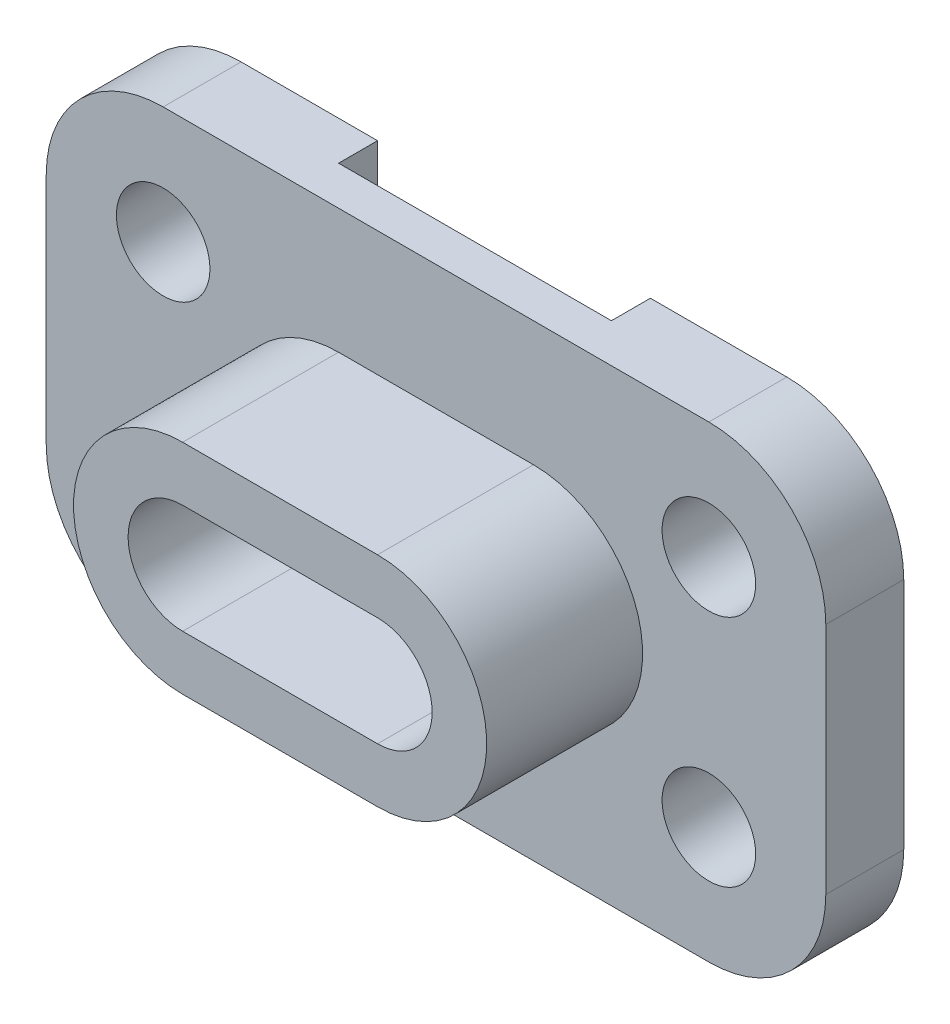
ISO-10303-21;
HEADER;
FILE_DESCRIPTION(('STEP AP214'),'2;1');
FILE_NAME('part.step','',(''),(''),'','','');
FILE_SCHEMA(('AUTOMOTIVE_DESIGN { 1 0 10303 214 1 1 1 1 }'));
ENDSEC;
DATA;
#1=APPLICATION_CONTEXT('core data for automotive mechanical design processes');
#2=APPLICATION_PROTOCOL_DEFINITION('international standard','automotive_design',2000,#1);
#3=PRODUCT_CONTEXT('',#1,'mechanical');
#4=PRODUCT('Part','Part','',(#3));
#5=PRODUCT_RELATED_PRODUCT_CATEGORY('part','',(#4));
#6=PRODUCT_DEFINITION_FORMATION('','',#4);
#7=PRODUCT_DEFINITION_CONTEXT('part definition',#1,'design');
#8=PRODUCT_DEFINITION('design','',#6,#7);
#9=PRODUCT_DEFINITION_SHAPE('','',#8);
#10=(LENGTH_UNIT() NAMED_UNIT(*) SI_UNIT(.MILLI.,.METRE.));
#11=(NAMED_UNIT(*) PLANE_ANGLE_UNIT() SI_UNIT($,.RADIAN.));
#12=(NAMED_UNIT(*) SI_UNIT($,.STERADIAN.) SOLID_ANGLE_UNIT());
#13=UNCERTAINTY_MEASURE_WITH_UNIT(LENGTH_MEASURE(1.E-05),#10,'distance_accuracy_value','');
#14=(GEOMETRIC_REPRESENTATION_CONTEXT(3) GLOBAL_UNCERTAINTY_ASSIGNED_CONTEXT((#13)) GLOBAL_UNIT_ASSIGNED_CONTEXT((#10,
#11,#12)) REPRESENTATION_CONTEXT('',''));
#15=CARTESIAN_POINT('',(0.,0.,0.));
#16=DIRECTION('',(0.,0.,1.));
#17=DIRECTION('',(1.,0.,0.));
#18=AXIS2_PLACEMENT_3D('',#15,#16,#17);
#19=CARTESIAN_POINT('',(15.,-45.,0.));
#20=DIRECTION('',(0.,0.,-1.));
#21=DIRECTION('',(-1.,0.,0.));
#22=AXIS2_PLACEMENT_3D('',#19,#20,#21);
#23=PLANE('',#22);
#24=DIRECTION('',(0.,-1.,0.));
#25=VECTOR('',#24,1.);
#26=CARTESIAN_POINT('',(32.5,0.,0.));
#27=LINE('',#26,#25);
#28=CARTESIAN_POINT('',(32.5,0.,0.));
#29=VERTEX_POINT('',#28);
#30=CARTESIAN_POINT('',(32.5,-60.,0.));
#31=VERTEX_POINT('',#30);
#32=EDGE_CURVE('E215',#29,#31,#27,.T.);
#33=ORIENTED_EDGE('',*,*,#32,.T.);
#34=DIRECTION('',(1.,0.,0.));
#35=VECTOR('',#34,1.);
#36=CARTESIAN_POINT('',(84.9999999999999,-60.,0.));
#37=LINE('',#36,#35);
#38=CARTESIAN_POINT('',(15.0000000000001,-60.,0.));
#39=VERTEX_POINT('',#38);
#40=EDGE_CURVE('E330',#39,#31,#37,.T.);
#41=ORIENTED_EDGE('',*,*,#40,.F.);
#42=CARTESIAN_POINT('',(15.,-45.,0.));
#43=DIRECTION('',(0.,0.,1.));
#44=DIRECTION('',(-1.,0.,0.));
#45=AXIS2_PLACEMENT_3D('',#42,#43,#44);
#46=CIRCLE('',#45,15.);
#47=CARTESIAN_POINT('',(0.,-44.9999999999999,0.));
#48=VERTEX_POINT('',#47);
#49=EDGE_CURVE('E304',#48,#39,#46,.T.);
#50=ORIENTED_EDGE('',*,*,#49,.F.);
#51=DIRECTION('',(0.,-1.,0.));
#52=VECTOR('',#51,1.);
#53=CARTESIAN_POINT('',(0.,-44.9999999999999,0.));
#54=LINE('',#53,#52);
#55=CARTESIAN_POINT('',(0.,-15.0000000000001,0.));
#56=VERTEX_POINT('',#55);
#57=EDGE_CURVE('E310',#56,#48,#54,.T.);
#58=ORIENTED_EDGE('',*,*,#57,.F.);
#59=CARTESIAN_POINT('',(15.,-15.,0.));
#60=DIRECTION('',(0.,0.,1.));
#61=DIRECTION('',(1.,0.,0.));
#62=AXIS2_PLACEMENT_3D('',#59,#60,#61);
#63=CIRCLE('',#62,15.);
#64=CARTESIAN_POINT('',(15.0000000000001,0.,0.));
#65=VERTEX_POINT('',#64);
#66=EDGE_CURVE('E336',#65,#56,#63,.T.);
#67=ORIENTED_EDGE('',*,*,#66,.F.);
#68=DIRECTION('',(-1.,0.,0.));
#69=VECTOR('',#68,1.);
#70=CARTESIAN_POINT('',(15.0000000000001,0.,0.));
#71=LINE('',#70,#69);
#72=EDGE_CURVE('E338',#29,#65,#71,.T.);
#73=ORIENTED_EDGE('',*,*,#72,.F.);
#74=EDGE_LOOP('',(#33,#41,#50,#58,#67,#73));
#75=FACE_BOUND('',#74,.T.);
#76=CARTESIAN_POINT('',(15.,-15.,0.));
#77=DIRECTION('',(0.,0.,1.));
#78=DIRECTION('',(1.,0.,0.));
#79=AXIS2_PLACEMENT_3D('',#76,#77,#78);
#80=CIRCLE('',#79,6.);
#81=CARTESIAN_POINT('',(21.,-15.,0.));
#82=VERTEX_POINT('',#81);
#83=EDGE_CURVE('E299',#82,#82,#80,.T.);
#84=ORIENTED_EDGE('',*,*,#83,.T.);
#85=EDGE_LOOP('',(#84));
#86=FACE_BOUND('',#85,.T.);
#87=CARTESIAN_POINT('',(15.,-45.,0.));
#88=DIRECTION('',(0.,0.,1.));
#89=DIRECTION('',(1.,0.,0.));
#90=AXIS2_PLACEMENT_3D('',#87,#88,#89);
#91=CIRCLE('',#90,6.);
#92=CARTESIAN_POINT('',(21.,-45.,0.));
#93=VERTEX_POINT('',#92);
#94=EDGE_CURVE('E294',#93,#93,#91,.T.);
#95=ORIENTED_EDGE('',*,*,#94,.T.);
#96=EDGE_LOOP('',(#95));
#97=FACE_BOUND('',#96,.T.);
#98=ADVANCED_FACE('F44',(#75,#86,#97),#23,.T.);
#99=CARTESIAN_POINT('',(15.,-45.,10.));
#100=DIRECTION('',(0.,0.,-1.));
#101=DIRECTION('',(-1.,0.,0.));
#102=AXIS2_PLACEMENT_3D('',#99,#100,#101);
#103=PLANE('',#102);
#104=CARTESIAN_POINT('',(15.,-45.,10.));
#105=DIRECTION('',(0.,0.,1.));
#106=DIRECTION('',(-1.,0.,0.));
#107=AXIS2_PLACEMENT_3D('',#104,#105,#106);
#108=CIRCLE('',#107,15.);
#109=CARTESIAN_POINT('',(0.,-44.9999999999999,10.));
#110=VERTEX_POINT('',#109);
#111=CARTESIAN_POINT('',(15.0000000000001,-60.,10.));
#112=VERTEX_POINT('',#111);
#113=EDGE_CURVE('E301',#110,#112,#108,.T.);
#114=ORIENTED_EDGE('',*,*,#113,.T.);
#115=DIRECTION('',(1.,0.,0.));
#116=VECTOR('',#115,1.);
#117=CARTESIAN_POINT('',(84.9999999999999,-60.,10.));
#118=LINE('',#117,#116);
#119=CARTESIAN_POINT('',(84.9999999999999,-60.,10.));
#120=VERTEX_POINT('',#119);
#121=EDGE_CURVE('E306',#112,#120,#118,.T.);
#122=ORIENTED_EDGE('',*,*,#121,.T.);
#123=CARTESIAN_POINT('',(85.,-45.,10.));
#124=DIRECTION('',(0.,0.,1.));
#125=DIRECTION('',(1.,0.,0.));
#126=AXIS2_PLACEMENT_3D('',#123,#124,#125);
#127=CIRCLE('',#126,15.);
#128=CARTESIAN_POINT('',(100.,-45.,10.));
#129=VERTEX_POINT('',#128);
#130=EDGE_CURVE('E313',#120,#129,#127,.T.);
#131=ORIENTED_EDGE('',*,*,#130,.T.);
#132=DIRECTION('',(0.,1.,0.));
#133=VECTOR('',#132,1.);
#134=CARTESIAN_POINT('',(100.,-15.0000000000001,10.));
#135=LINE('',#134,#133);
#136=CARTESIAN_POINT('',(100.,-15.0000000000001,10.));
#137=VERTEX_POINT('',#136);
#138=EDGE_CURVE('E311',#129,#137,#135,.T.);
#139=ORIENTED_EDGE('',*,*,#138,.T.);
#140=CARTESIAN_POINT('',(85.,-15.,10.));
#141=DIRECTION('',(0.,0.,1.));
#142=DIRECTION('',(1.,0.,0.));
#143=AXIS2_PLACEMENT_3D('',#140,#141,#142);
#144=CIRCLE('',#143,15.);
#145=CARTESIAN_POINT('',(84.9999999999999,0.,10.));
#146=VERTEX_POINT('',#145);
#147=EDGE_CURVE('E312',#137,#146,#144,.T.);
#148=ORIENTED_EDGE('',*,*,#147,.T.);
#149=DIRECTION('',(-1.,0.,0.));
#150=VECTOR('',#149,1.);
#151=CARTESIAN_POINT('',(15.0000000000001,0.,10.));
#152=LINE('',#151,#150);
#153=CARTESIAN_POINT('',(15.0000000000001,0.,10.));
#154=VERTEX_POINT('',#153);
#155=EDGE_CURVE('E320',#146,#154,#152,.T.);
#156=ORIENTED_EDGE('',*,*,#155,.T.);
#157=CARTESIAN_POINT('',(15.,-15.,10.));
#158=DIRECTION('',(0.,0.,1.));
#159=DIRECTION('',(1.,0.,0.));
#160=AXIS2_PLACEMENT_3D('',#157,#158,#159);
#161=CIRCLE('',#160,15.);
#162=CARTESIAN_POINT('',(0.,-15.0000000000001,10.));
#163=VERTEX_POINT('',#162);
#164=EDGE_CURVE('E317',#154,#163,#161,.T.);
#165=ORIENTED_EDGE('',*,*,#164,.T.);
#166=DIRECTION('',(0.,-1.,0.));
#167=VECTOR('',#166,1.);
#168=CARTESIAN_POINT('',(0.,-44.9999999999999,10.));
#169=LINE('',#168,#167);
#170=EDGE_CURVE('E321',#163,#110,#169,.T.);
#171=ORIENTED_EDGE('',*,*,#170,.T.);
#172=EDGE_LOOP('',(#114,#122,#131,#139,#148,#156,#165,#171));
#173=FACE_BOUND('',#172,.T.);
#174=CARTESIAN_POINT('',(15.,-15.,10.));
#175=DIRECTION('',(0.,0.,1.));
#176=DIRECTION('',(1.,0.,0.));
#177=AXIS2_PLACEMENT_3D('',#174,#175,#176);
#178=CIRCLE('',#177,6.);
#179=CARTESIAN_POINT('',(21.,-15.,10.));
#180=VERTEX_POINT('',#179);
#181=EDGE_CURVE('E284',#180,#180,#178,.T.);
#182=ORIENTED_EDGE('',*,*,#181,.F.);
#183=EDGE_LOOP('',(#182));
#184=FACE_BOUND('',#183,.T.);
#185=CARTESIAN_POINT('',(85.,-15.,10.));
#186=DIRECTION('',(0.,0.,1.));
#187=DIRECTION('',(1.,0.,0.));
#188=AXIS2_PLACEMENT_3D('',#185,#186,#187);
#189=CIRCLE('',#188,6.);
#190=CARTESIAN_POINT('',(91.,-15.,10.));
#191=VERTEX_POINT('',#190);
#192=EDGE_CURVE('E282',#191,#191,#189,.T.);
#193=ORIENTED_EDGE('',*,*,#192,.F.);
#194=EDGE_LOOP('',(#193));
#195=FACE_BOUND('',#194,.T.);
#196=CARTESIAN_POINT('',(85.,-45.,10.));
#197=DIRECTION('',(0.,0.,1.));
#198=DIRECTION('',(1.,0.,0.));
#199=AXIS2_PLACEMENT_3D('',#196,#197,#198);
#200=CIRCLE('',#199,6.);
#201=CARTESIAN_POINT('',(91.,-45.,10.));
#202=VERTEX_POINT('',#201);
#203=EDGE_CURVE('E292',#202,#202,#200,.T.);
#204=ORIENTED_EDGE('',*,*,#203,.F.);
#205=EDGE_LOOP('',(#204));
#206=FACE_BOUND('',#205,.T.);
#207=CARTESIAN_POINT('',(15.,-45.,10.));
#208=DIRECTION('',(0.,0.,1.));
#209=DIRECTION('',(1.,0.,0.));
#210=AXIS2_PLACEMENT_3D('',#207,#208,#209);
#211=CIRCLE('',#210,6.);
#212=CARTESIAN_POINT('',(21.,-45.,10.));
#213=VERTEX_POINT('',#212);
#214=EDGE_CURVE('E278',#213,#213,#211,.T.);
#215=ORIENTED_EDGE('',*,*,#214,.F.);
#216=EDGE_LOOP('',(#215));
#217=FACE_BOUND('',#216,.T.);
#218=CARTESIAN_POINT('',(37.5,-30.,10.));
#219=DIRECTION('',(0.,0.,1.));
#220=DIRECTION('',(1.,0.,0.));
#221=AXIS2_PLACEMENT_3D('',#218,#219,#220);
#222=CIRCLE('',#221,14.);
#223=CARTESIAN_POINT('',(37.5,-16.,10.));
#224=VERTEX_POINT('',#223);
#225=CARTESIAN_POINT('',(37.5,-44.,10.));
#226=VERTEX_POINT('',#225);
#227=EDGE_CURVE('E245',#224,#226,#222,.T.);
#228=ORIENTED_EDGE('',*,*,#227,.F.);
#229=DIRECTION('',(-1.,0.,0.));
#230=VECTOR('',#229,1.);
#231=CARTESIAN_POINT('',(37.5,-16.,10.));
#232=LINE('',#231,#230);
#233=CARTESIAN_POINT('',(62.5,-16.,10.));
#234=VERTEX_POINT('',#233);
#235=EDGE_CURVE('E252',#234,#224,#232,.T.);
#236=ORIENTED_EDGE('',*,*,#235,.F.);
#237=CARTESIAN_POINT('',(62.5,-30.,10.));
#238=DIRECTION('',(0.,0.,1.));
#239=DIRECTION('',(1.,0.,0.));
#240=AXIS2_PLACEMENT_3D('',#237,#238,#239);
#241=CIRCLE('',#240,14.);
#242=CARTESIAN_POINT('',(62.5,-44.,10.));
#243=VERTEX_POINT('',#242);
#244=EDGE_CURVE('E262',#243,#234,#241,.T.);
#245=ORIENTED_EDGE('',*,*,#244,.F.);
#246=DIRECTION('',(1.,0.,0.));
#247=VECTOR('',#246,1.);
#248=CARTESIAN_POINT('',(62.5,-44.,10.));
#249=LINE('',#248,#247);
#250=EDGE_CURVE('E261',#226,#243,#249,.T.);
#251=ORIENTED_EDGE('',*,*,#250,.F.);
#252=EDGE_LOOP('',(#228,#236,#245,#251));
#253=FACE_BOUND('',#252,.T.);
#254=ADVANCED_FACE('F379',(#173,#184,#195,#206,#217,#253),#103,.F.);
#255=CARTESIAN_POINT('',(15.,-45.,10.));
#256=DIRECTION('',(0.,0.,-1.));
#257=DIRECTION('',(-1.,0.,0.));
#258=AXIS2_PLACEMENT_3D('',#255,#256,#257);
#259=CYLINDRICAL_SURFACE('',#258,15.);
#260=ORIENTED_EDGE('',*,*,#49,.T.);
#261=DIRECTION('',(0.,0.,-1.));
#262=VECTOR('',#261,1.);
#263=CARTESIAN_POINT('',(15.0000000000001,-60.,10.));
#264=LINE('',#263,#262);
#265=EDGE_CURVE('E11',#112,#39,#264,.T.);
#266=ORIENTED_EDGE('',*,*,#265,.F.);
#267=ORIENTED_EDGE('',*,*,#113,.F.);
#268=DIRECTION('',(0.,0.,-1.));
#269=VECTOR('',#268,1.);
#270=CARTESIAN_POINT('',(0.,-44.9999999999999,10.));
#271=LINE('',#270,#269);
#272=EDGE_CURVE('E323',#110,#48,#271,.T.);
#273=ORIENTED_EDGE('',*,*,#272,.T.);
#274=EDGE_LOOP('',(#260,#266,#267,#273));
#275=FACE_BOUND('',#274,.T.);
#276=ADVANCED_FACE('F50',(#275),#259,.T.);
#277=CARTESIAN_POINT('',(84.9999999999999,-60.,10.));
#278=DIRECTION('',(0.,1.,0.));
#279=DIRECTION('',(0.,0.,1.));
#280=AXIS2_PLACEMENT_3D('',#277,#278,#279);
#281=PLANE('',#280);
#282=ORIENTED_EDGE('',*,*,#40,.T.);
#283=DIRECTION('',(0.,0.,-1.));
#284=VECTOR('',#283,1.);
#285=CARTESIAN_POINT('',(32.5,-60.,5.));
#286=LINE('',#285,#284);
#287=CARTESIAN_POINT('',(32.5,-60.,5.));
#288=VERTEX_POINT('',#287);
#289=EDGE_CURVE('E204',#288,#31,#286,.T.);
#290=ORIENTED_EDGE('',*,*,#289,.F.);
#291=DIRECTION('',(-1.,0.,0.));
#292=VECTOR('',#291,1.);
#293=CARTESIAN_POINT('',(67.5,-60.,5.));
#294=LINE('',#293,#292);
#295=CARTESIAN_POINT('',(67.5,-60.,5.));
#296=VERTEX_POINT('',#295);
#297=EDGE_CURVE('E206',#296,#288,#294,.T.);
#298=ORIENTED_EDGE('',*,*,#297,.F.);
#299=DIRECTION('',(0.,0.,1.));
#300=VECTOR('',#299,1.);
#301=CARTESIAN_POINT('',(67.5,-60.,0.));
#302=LINE('',#301,#300);
#303=CARTESIAN_POINT('',(67.5,-60.,0.));
#304=VERTEX_POINT('',#303);
#305=EDGE_CURVE('E184',#304,#296,#302,.T.);
#306=ORIENTED_EDGE('',*,*,#305,.F.);
#307=CARTESIAN_POINT('',(84.9999999999999,-60.,0.));
#308=VERTEX_POINT('',#307);
#309=EDGE_CURVE('E326',#304,#308,#37,.T.);
#310=ORIENTED_EDGE('',*,*,#309,.T.);
#311=DIRECTION('',(0.,0.,-1.));
#312=VECTOR('',#311,1.);
#313=CARTESIAN_POINT('',(84.9999999999999,-60.,10.));
#314=LINE('',#313,#312);
#315=EDGE_CURVE('E52',#120,#308,#314,.T.);
#316=ORIENTED_EDGE('',*,*,#315,.F.);
#317=ORIENTED_EDGE('',*,*,#121,.F.);
#318=ORIENTED_EDGE('',*,*,#265,.T.);
#319=EDGE_LOOP('',(#282,#290,#298,#306,#310,#316,#317,#318));
#320=FACE_BOUND('',#319,.T.);
#321=ADVANCED_FACE('F384',(#320),#281,.F.);
#322=CARTESIAN_POINT('',(85.,-45.,10.));
#323=DIRECTION('',(0.,0.,-1.));
#324=DIRECTION('',(-1.,0.,0.));
#325=AXIS2_PLACEMENT_3D('',#322,#323,#324);
#326=CYLINDRICAL_SURFACE('',#325,15.);
#327=CARTESIAN_POINT('',(85.,-45.,0.));
#328=DIRECTION('',(0.,0.,1.));
#329=DIRECTION('',(1.,0.,0.));
#330=AXIS2_PLACEMENT_3D('',#327,#328,#329);
#331=CIRCLE('',#330,15.);
#332=CARTESIAN_POINT('',(100.,-45.,0.));
#333=VERTEX_POINT('',#332);
#334=EDGE_CURVE('E329',#308,#333,#331,.T.);
#335=ORIENTED_EDGE('',*,*,#334,.T.);
#336=DIRECTION('',(0.,0.,-1.));
#337=VECTOR('',#336,1.);
#338=CARTESIAN_POINT('',(100.,-45.,10.));
#339=LINE('',#338,#337);
#340=EDGE_CURVE('E354',#129,#333,#339,.T.);
#341=ORIENTED_EDGE('',*,*,#340,.F.);
#342=ORIENTED_EDGE('',*,*,#130,.F.);
#343=ORIENTED_EDGE('',*,*,#315,.T.);
#344=EDGE_LOOP('',(#335,#341,#342,#343));
#345=FACE_BOUND('',#344,.T.);
#346=ADVANCED_FACE('F363',(#345),#326,.T.);
#347=CARTESIAN_POINT('',(100.,-15.0000000000001,10.));
#348=DIRECTION('',(-1.,0.,0.));
#349=DIRECTION('',(0.,0.,1.));
#350=AXIS2_PLACEMENT_3D('',#347,#348,#349);
#351=PLANE('',#350);
#352=DIRECTION('',(0.,1.,0.));
#353=VECTOR('',#352,1.);
#354=CARTESIAN_POINT('',(100.,-15.0000000000001,0.));
#355=LINE('',#354,#353);
#356=CARTESIAN_POINT('',(100.,-15.0000000000001,0.));
#357=VERTEX_POINT('',#356);
#358=EDGE_CURVE('E335',#333,#357,#355,.T.);
#359=ORIENTED_EDGE('',*,*,#358,.T.);
#360=DIRECTION('',(0.,0.,-1.));
#361=VECTOR('',#360,1.);
#362=CARTESIAN_POINT('',(100.,-15.0000000000001,10.));
#363=LINE('',#362,#361);
#364=EDGE_CURVE('E353',#137,#357,#363,.T.);
#365=ORIENTED_EDGE('',*,*,#364,.F.);
#366=ORIENTED_EDGE('',*,*,#138,.F.);
#367=ORIENTED_EDGE('',*,*,#340,.T.);
#368=EDGE_LOOP('',(#359,#365,#366,#367));
#369=FACE_BOUND('',#368,.T.);
#370=ADVANCED_FACE('F375',(#369),#351,.F.);
#371=CARTESIAN_POINT('',(85.,-15.,10.));
#372=DIRECTION('',(0.,0.,-1.));
#373=DIRECTION('',(-1.,0.,0.));
#374=AXIS2_PLACEMENT_3D('',#371,#372,#373);
#375=CYLINDRICAL_SURFACE('',#374,15.);
#376=CARTESIAN_POINT('',(85.,-15.,0.));
#377=DIRECTION('',(0.,0.,1.));
#378=DIRECTION('',(1.,0.,0.));
#379=AXIS2_PLACEMENT_3D('',#376,#377,#378);
#380=CIRCLE('',#379,15.);
#381=CARTESIAN_POINT('',(84.9999999999999,0.,0.));
#382=VERTEX_POINT('',#381);
#383=EDGE_CURVE('E331',#357,#382,#380,.T.);
#384=ORIENTED_EDGE('',*,*,#383,.T.);
#385=DIRECTION('',(0.,0.,-1.));
#386=VECTOR('',#385,1.);
#387=CARTESIAN_POINT('',(84.9999999999999,0.,10.));
#388=LINE('',#387,#386);
#389=EDGE_CURVE('E349',#146,#382,#388,.T.);
#390=ORIENTED_EDGE('',*,*,#389,.F.);
#391=ORIENTED_EDGE('',*,*,#147,.F.);
#392=ORIENTED_EDGE('',*,*,#364,.T.);
#393=EDGE_LOOP('',(#384,#390,#391,#392));
#394=FACE_BOUND('',#393,.T.);
#395=ADVANCED_FACE('F376',(#394),#375,.T.);
#396=CARTESIAN_POINT('',(15.0000000000001,0.,10.));
#397=DIRECTION('',(0.,-1.,0.));
#398=DIRECTION('',(0.,0.,-1.));
#399=AXIS2_PLACEMENT_3D('',#396,#397,#398);
#400=PLANE('',#399);
#401=DIRECTION('',(-1.,0.,0.));
#402=VECTOR('',#401,1.);
#403=CARTESIAN_POINT('',(67.5,0.,5.));
#404=LINE('',#403,#402);
#405=CARTESIAN_POINT('',(67.5,0.,5.));
#406=VERTEX_POINT('',#405);
#407=CARTESIAN_POINT('',(32.5,0.,5.));
#408=VERTEX_POINT('',#407);
#409=EDGE_CURVE('E194',#406,#408,#404,.T.);
#410=ORIENTED_EDGE('',*,*,#409,.T.);
#411=DIRECTION('',(0.,0.,-1.));
#412=VECTOR('',#411,1.);
#413=CARTESIAN_POINT('',(32.5,0.,5.));
#414=LINE('',#413,#412);
#415=EDGE_CURVE('E197',#408,#29,#414,.T.);
#416=ORIENTED_EDGE('',*,*,#415,.T.);
#417=ORIENTED_EDGE('',*,*,#72,.T.);
#418=DIRECTION('',(0.,0.,-1.));
#419=VECTOR('',#418,1.);
#420=CARTESIAN_POINT('',(15.0000000000001,0.,10.));
#421=LINE('',#420,#419);
#422=EDGE_CURVE('E347',#154,#65,#421,.T.);
#423=ORIENTED_EDGE('',*,*,#422,.F.);
#424=ORIENTED_EDGE('',*,*,#155,.F.);
#425=ORIENTED_EDGE('',*,*,#389,.T.);
#426=CARTESIAN_POINT('',(67.5,0.,0.));
#427=VERTEX_POINT('',#426);
#428=EDGE_CURVE('E201',#382,#427,#71,.T.);
#429=ORIENTED_EDGE('',*,*,#428,.T.);
#430=DIRECTION('',(0.,0.,1.));
#431=VECTOR('',#430,1.);
#432=CARTESIAN_POINT('',(67.5,0.,0.));
#433=LINE('',#432,#431);
#434=EDGE_CURVE('E58',#427,#406,#433,.T.);
#435=ORIENTED_EDGE('',*,*,#434,.T.);
#436=EDGE_LOOP('',(#410,#416,#417,#423,#424,#425,#429,#435));
#437=FACE_BOUND('',#436,.T.);
#438=ADVANCED_FACE('F199',(#437),#400,.F.);
#439=CARTESIAN_POINT('',(15.,-15.,10.));
#440=DIRECTION('',(0.,0.,-1.));
#441=DIRECTION('',(-1.,0.,0.));
#442=AXIS2_PLACEMENT_3D('',#439,#440,#441);
#443=CYLINDRICAL_SURFACE('',#442,15.);
#444=ORIENTED_EDGE('',*,*,#66,.T.);
#445=DIRECTION('',(0.,0.,-1.));
#446=VECTOR('',#445,1.);
#447=CARTESIAN_POINT('',(0.,-15.0000000000001,10.));
#448=LINE('',#447,#446);
#449=EDGE_CURVE('E342',#163,#56,#448,.T.);
#450=ORIENTED_EDGE('',*,*,#449,.F.);
#451=ORIENTED_EDGE('',*,*,#164,.F.);
#452=ORIENTED_EDGE('',*,*,#422,.T.);
#453=EDGE_LOOP('',(#444,#450,#451,#452));
#454=FACE_BOUND('',#453,.T.);
#455=ADVANCED_FACE('F400',(#454),#443,.T.);
#456=CARTESIAN_POINT('',(0.,-44.9999999999999,10.));
#457=DIRECTION('',(1.,0.,0.));
#458=DIRECTION('',(0.,0.,-1.));
#459=AXIS2_PLACEMENT_3D('',#456,#457,#458);
#460=PLANE('',#459);
#461=ORIENTED_EDGE('',*,*,#57,.T.);
#462=ORIENTED_EDGE('',*,*,#272,.F.);
#463=ORIENTED_EDGE('',*,*,#170,.F.);
#464=ORIENTED_EDGE('',*,*,#449,.T.);
#465=EDGE_LOOP('',(#461,#462,#463,#464));
#466=FACE_BOUND('',#465,.T.);
#467=ADVANCED_FACE('F401',(#466),#460,.F.);
#468=DIRECTION('',(0.,-1.,0.));
#469=VECTOR('',#468,1.);
#470=CARTESIAN_POINT('',(67.5,0.,0.));
#471=LINE('',#470,#469);
#472=EDGE_CURVE('E189',#427,#304,#471,.T.);
#473=ORIENTED_EDGE('',*,*,#472,.F.);
#474=ORIENTED_EDGE('',*,*,#428,.F.);
#475=ORIENTED_EDGE('',*,*,#383,.F.);
#476=ORIENTED_EDGE('',*,*,#358,.F.);
#477=ORIENTED_EDGE('',*,*,#334,.F.);
#478=ORIENTED_EDGE('',*,*,#309,.F.);
#479=EDGE_LOOP('',(#473,#474,#475,#476,#477,#478));
#480=FACE_BOUND('',#479,.T.);
#481=CARTESIAN_POINT('',(85.,-45.,0.));
#482=DIRECTION('',(0.,0.,1.));
#483=DIRECTION('',(1.,0.,0.));
#484=AXIS2_PLACEMENT_3D('',#481,#482,#483);
#485=CIRCLE('',#484,6.);
#486=CARTESIAN_POINT('',(91.,-45.,0.));
#487=VERTEX_POINT('',#486);
#488=EDGE_CURVE('E287',#487,#487,#485,.T.);
#489=ORIENTED_EDGE('',*,*,#488,.T.);
#490=EDGE_LOOP('',(#489));
#491=FACE_BOUND('',#490,.T.);
#492=CARTESIAN_POINT('',(85.,-15.,0.));
#493=DIRECTION('',(0.,0.,1.));
#494=DIRECTION('',(1.,0.,0.));
#495=AXIS2_PLACEMENT_3D('',#492,#493,#494);
#496=CIRCLE('',#495,6.);
#497=CARTESIAN_POINT('',(91.,-15.,0.));
#498=VERTEX_POINT('',#497);
#499=EDGE_CURVE('E283',#498,#498,#496,.T.);
#500=ORIENTED_EDGE('',*,*,#499,.T.);
#501=EDGE_LOOP('',(#500));
#502=FACE_BOUND('',#501,.T.);
#503=ADVANCED_FACE('F370',(#480,#491,#502),#23,.T.);
#504=CARTESIAN_POINT('',(15.,-15.,0.));
#505=DIRECTION('',(0.,0.,1.));
#506=DIRECTION('',(1.,0.,0.));
#507=AXIS2_PLACEMENT_3D('',#504,#505,#506);
#508=CYLINDRICAL_SURFACE('',#507,6.);
#509=ORIENTED_EDGE('',*,*,#83,.F.);
#510=EDGE_LOOP('',(#509));
#511=FACE_BOUND('',#510,.T.);
#512=ORIENTED_EDGE('',*,*,#181,.T.);
#513=EDGE_LOOP('',(#512));
#514=FACE_BOUND('',#513,.T.);
#515=ADVANCED_FACE('F413',(#511,#514),#508,.F.);
#516=CARTESIAN_POINT('',(85.,-15.,0.));
#517=DIRECTION('',(0.,0.,1.));
#518=DIRECTION('',(1.,0.,0.));
#519=AXIS2_PLACEMENT_3D('',#516,#517,#518);
#520=CYLINDRICAL_SURFACE('',#519,6.);
#521=ORIENTED_EDGE('',*,*,#499,.F.);
#522=EDGE_LOOP('',(#521));
#523=FACE_BOUND('',#522,.T.);
#524=ORIENTED_EDGE('',*,*,#192,.T.);
#525=EDGE_LOOP('',(#524));
#526=FACE_BOUND('',#525,.T.);
#527=ADVANCED_FACE('F424',(#523,#526),#520,.F.);
#528=CARTESIAN_POINT('',(85.,-45.,0.));
#529=DIRECTION('',(0.,0.,1.));
#530=DIRECTION('',(1.,0.,0.));
#531=AXIS2_PLACEMENT_3D('',#528,#529,#530);
#532=CYLINDRICAL_SURFACE('',#531,6.);
#533=ORIENTED_EDGE('',*,*,#488,.F.);
#534=EDGE_LOOP('',(#533));
#535=FACE_BOUND('',#534,.T.);
#536=ORIENTED_EDGE('',*,*,#203,.T.);
#537=EDGE_LOOP('',(#536));
#538=FACE_BOUND('',#537,.T.);
#539=ADVANCED_FACE('F429',(#535,#538),#532,.F.);
#540=CARTESIAN_POINT('',(15.,-45.,0.));
#541=DIRECTION('',(0.,0.,1.));
#542=DIRECTION('',(1.,0.,0.));
#543=AXIS2_PLACEMENT_3D('',#540,#541,#542);
#544=CYLINDRICAL_SURFACE('',#543,6.);
#545=ORIENTED_EDGE('',*,*,#94,.F.);
#546=EDGE_LOOP('',(#545));
#547=FACE_BOUND('',#546,.T.);
#548=ORIENTED_EDGE('',*,*,#214,.T.);
#549=EDGE_LOOP('',(#548));
#550=FACE_BOUND('',#549,.T.);
#551=ADVANCED_FACE('F426',(#547,#550),#544,.F.);
#552=CARTESIAN_POINT('',(37.5,-30.,30.));
#553=DIRECTION('',(0.,0.,-1.));
#554=DIRECTION('',(-1.,0.,0.));
#555=AXIS2_PLACEMENT_3D('',#552,#553,#554);
#556=CYLINDRICAL_SURFACE('',#555,14.);
#557=ORIENTED_EDGE('',*,*,#227,.T.);
#558=DIRECTION('',(0.,0.,-1.));
#559=VECTOR('',#558,1.);
#560=CARTESIAN_POINT('',(37.5,-44.,30.));
#561=LINE('',#560,#559);
#562=CARTESIAN_POINT('',(37.5,-44.,30.));
#563=VERTEX_POINT('',#562);
#564=EDGE_CURVE('E280',#563,#226,#561,.T.);
#565=ORIENTED_EDGE('',*,*,#564,.F.);
#566=CARTESIAN_POINT('',(37.5,-30.,30.));
#567=DIRECTION('',(0.,0.,1.));
#568=DIRECTION('',(1.,0.,0.));
#569=AXIS2_PLACEMENT_3D('',#566,#567,#568);
#570=CIRCLE('',#569,14.);
#571=CARTESIAN_POINT('',(37.5,-16.,30.));
#572=VERTEX_POINT('',#571);
#573=EDGE_CURVE('E247',#572,#563,#570,.T.);
#574=ORIENTED_EDGE('',*,*,#573,.F.);
#575=DIRECTION('',(0.,0.,-1.));
#576=VECTOR('',#575,1.);
#577=CARTESIAN_POINT('',(37.5,-16.,30.));
#578=LINE('',#577,#576);
#579=EDGE_CURVE('E256',#572,#224,#578,.T.);
#580=ORIENTED_EDGE('',*,*,#579,.T.);
#581=EDGE_LOOP('',(#557,#565,#574,#580));
#582=FACE_BOUND('',#581,.T.);
#583=ADVANCED_FACE('F427',(#582),#556,.T.);
#584=CARTESIAN_POINT('',(62.5,-44.,30.));
#585=DIRECTION('',(0.,1.,0.));
#586=DIRECTION('',(0.,0.,1.));
#587=AXIS2_PLACEMENT_3D('',#584,#585,#586);
#588=PLANE('',#587);
#589=ORIENTED_EDGE('',*,*,#250,.T.);
#590=DIRECTION('',(0.,0.,-1.));
#591=VECTOR('',#590,1.);
#592=CARTESIAN_POINT('',(62.5,-44.,30.));
#593=LINE('',#592,#591);
#594=CARTESIAN_POINT('',(62.5,-44.,30.));
#595=VERTEX_POINT('',#594);
#596=EDGE_CURVE('E273',#595,#243,#593,.T.);
#597=ORIENTED_EDGE('',*,*,#596,.F.);
#598=DIRECTION('',(1.,0.,0.));
#599=VECTOR('',#598,1.);
#600=CARTESIAN_POINT('',(62.5,-44.,30.));
#601=LINE('',#600,#599);
#602=EDGE_CURVE('E253',#563,#595,#601,.T.);
#603=ORIENTED_EDGE('',*,*,#602,.F.);
#604=ORIENTED_EDGE('',*,*,#564,.T.);
#605=EDGE_LOOP('',(#589,#597,#603,#604));
#606=FACE_BOUND('',#605,.T.);
#607=ADVANCED_FACE('F439',(#606),#588,.F.);
#608=CARTESIAN_POINT('',(62.5,-30.,30.));
#609=DIRECTION('',(0.,0.,-1.));
#610=DIRECTION('',(-1.,0.,0.));
#611=AXIS2_PLACEMENT_3D('',#608,#609,#610);
#612=CYLINDRICAL_SURFACE('',#611,14.);
#613=ORIENTED_EDGE('',*,*,#244,.T.);
#614=DIRECTION('',(0.,0.,-1.));
#615=VECTOR('',#614,1.);
#616=CARTESIAN_POINT('',(62.5,-16.,30.));
#617=LINE('',#616,#615);
#618=CARTESIAN_POINT('',(62.5,-16.,30.));
#619=VERTEX_POINT('',#618);
#620=EDGE_CURVE('E271',#619,#234,#617,.T.);
#621=ORIENTED_EDGE('',*,*,#620,.F.);
#622=CARTESIAN_POINT('',(62.5,-30.,30.));
#623=DIRECTION('',(0.,0.,1.));
#624=DIRECTION('',(1.,0.,0.));
#625=AXIS2_PLACEMENT_3D('',#622,#623,#624);
#626=CIRCLE('',#625,14.);
#627=EDGE_CURVE('E255',#595,#619,#626,.T.);
#628=ORIENTED_EDGE('',*,*,#627,.F.);
#629=ORIENTED_EDGE('',*,*,#596,.T.);
#630=EDGE_LOOP('',(#613,#621,#628,#629));
#631=FACE_BOUND('',#630,.T.);
#632=ADVANCED_FACE('F441',(#631),#612,.T.);
#633=CARTESIAN_POINT('',(37.5,-16.,30.));
#634=DIRECTION('',(0.,-1.,0.));
#635=DIRECTION('',(0.,0.,-1.));
#636=AXIS2_PLACEMENT_3D('',#633,#634,#635);
#637=PLANE('',#636);
#638=ORIENTED_EDGE('',*,*,#235,.T.);
#639=ORIENTED_EDGE('',*,*,#579,.F.);
#640=DIRECTION('',(-1.,0.,0.));
#641=VECTOR('',#640,1.);
#642=CARTESIAN_POINT('',(37.5,-16.,30.));
#643=LINE('',#642,#641);
#644=EDGE_CURVE('E258',#619,#572,#643,.T.);
#645=ORIENTED_EDGE('',*,*,#644,.F.);
#646=ORIENTED_EDGE('',*,*,#620,.T.);
#647=EDGE_LOOP('',(#638,#639,#645,#646));
#648=FACE_BOUND('',#647,.T.);
#649=ADVANCED_FACE('F446',(#648),#637,.F.);
#650=CARTESIAN_POINT('',(37.5,-30.,30.));
#651=DIRECTION('',(0.,0.,1.));
#652=DIRECTION('',(1.,0.,0.));
#653=AXIS2_PLACEMENT_3D('',#650,#651,#652);
#654=PLANE('',#653);
#655=CARTESIAN_POINT('',(37.5,-30.,30.));
#656=DIRECTION('',(0.,0.,1.));
#657=DIRECTION('',(1.,0.,0.));
#658=AXIS2_PLACEMENT_3D('',#655,#656,#657);
#659=CIRCLE('',#658,7.);
#660=CARTESIAN_POINT('',(37.5,-23.0000000000001,30.));
#661=VERTEX_POINT('',#660);
#662=CARTESIAN_POINT('',(37.5,-37.0000000000001,30.));
#663=VERTEX_POINT('',#662);
#664=EDGE_CURVE('E67',#661,#663,#659,.T.);
#665=ORIENTED_EDGE('',*,*,#664,.F.);
#666=DIRECTION('',(-1.,0.,0.));
#667=VECTOR('',#666,1.);
#668=CARTESIAN_POINT('',(37.5,-23.0000000000001,30.));
#669=LINE('',#668,#667);
#670=CARTESIAN_POINT('',(62.5,-23.0000000000001,30.));
#671=VERTEX_POINT('',#670);
#672=EDGE_CURVE('E222',#671,#661,#669,.T.);
#673=ORIENTED_EDGE('',*,*,#672,.F.);
#674=CARTESIAN_POINT('',(62.5,-30.,30.));
#675=DIRECTION('',(0.,0.,1.));
#676=DIRECTION('',(1.,0.,0.));
#677=AXIS2_PLACEMENT_3D('',#674,#675,#676);
#678=CIRCLE('',#677,7.);
#679=CARTESIAN_POINT('',(62.5,-37.0000000000001,30.));
#680=VERTEX_POINT('',#679);
#681=EDGE_CURVE('E231',#680,#671,#678,.T.);
#682=ORIENTED_EDGE('',*,*,#681,.F.);
#683=DIRECTION('',(1.,0.,0.));
#684=VECTOR('',#683,1.);
#685=CARTESIAN_POINT('',(62.5,-37.0000000000001,30.));
#686=LINE('',#685,#684);
#687=EDGE_CURVE('E234',#663,#680,#686,.T.);
#688=ORIENTED_EDGE('',*,*,#687,.F.);
#689=EDGE_LOOP('',(#665,#673,#682,#688));
#690=FACE_BOUND('',#689,.T.);
#691=ORIENTED_EDGE('',*,*,#573,.T.);
#692=ORIENTED_EDGE('',*,*,#602,.T.);
#693=ORIENTED_EDGE('',*,*,#627,.T.);
#694=ORIENTED_EDGE('',*,*,#644,.T.);
#695=EDGE_LOOP('',(#691,#692,#693,#694));
#696=FACE_BOUND('',#695,.T.);
#697=ADVANCED_FACE('F454',(#690,#696),#654,.T.);
#698=CARTESIAN_POINT('',(37.5,-30.,10.));
#699=DIRECTION('',(0.,0.,1.));
#700=DIRECTION('',(1.,0.,0.));
#701=AXIS2_PLACEMENT_3D('',#698,#699,#700);
#702=CYLINDRICAL_SURFACE('',#701,7.);
#703=ORIENTED_EDGE('',*,*,#664,.T.);
#704=DIRECTION('',(0.,0.,1.));
#705=VECTOR('',#704,1.);
#706=CARTESIAN_POINT('',(37.5,-37.0000000000001,10.));
#707=LINE('',#706,#705);
#708=CARTESIAN_POINT('',(37.5,-37.0000000000001,10.));
#709=VERTEX_POINT('',#708);
#710=EDGE_CURVE('E227',#709,#663,#707,.T.);
#711=ORIENTED_EDGE('',*,*,#710,.F.);
#712=CARTESIAN_POINT('',(37.5,-30.,10.));
#713=DIRECTION('',(0.,0.,1.));
#714=DIRECTION('',(1.,0.,0.));
#715=AXIS2_PLACEMENT_3D('',#712,#713,#714);
#716=CIRCLE('',#715,7.);
#717=CARTESIAN_POINT('',(37.5,-23.0000000000001,10.));
#718=VERTEX_POINT('',#717);
#719=EDGE_CURVE('E220',#718,#709,#716,.T.);
#720=ORIENTED_EDGE('',*,*,#719,.F.);
#721=DIRECTION('',(0.,0.,1.));
#722=VECTOR('',#721,1.);
#723=CARTESIAN_POINT('',(37.5,-23.0000000000001,10.));
#724=LINE('',#723,#722);
#725=EDGE_CURVE('E238',#718,#661,#724,.T.);
#726=ORIENTED_EDGE('',*,*,#725,.T.);
#727=EDGE_LOOP('',(#703,#711,#720,#726));
#728=FACE_BOUND('',#727,.T.);
#729=ADVANCED_FACE('F457',(#728),#702,.F.);
#730=CARTESIAN_POINT('',(37.5,-23.0000000000001,10.));
#731=DIRECTION('',(0.,1.,0.));
#732=DIRECTION('',(0.,0.,1.));
#733=AXIS2_PLACEMENT_3D('',#730,#731,#732);
#734=PLANE('',#733);
#735=ORIENTED_EDGE('',*,*,#672,.T.);
#736=ORIENTED_EDGE('',*,*,#725,.F.);
#737=DIRECTION('',(-1.,0.,0.));
#738=VECTOR('',#737,1.);
#739=CARTESIAN_POINT('',(37.5,-23.0000000000001,10.));
#740=LINE('',#739,#738);
#741=CARTESIAN_POINT('',(62.5,-23.0000000000001,10.));
#742=VERTEX_POINT('',#741);
#743=EDGE_CURVE('E230',#742,#718,#740,.T.);
#744=ORIENTED_EDGE('',*,*,#743,.F.);
#745=DIRECTION('',(0.,0.,1.));
#746=VECTOR('',#745,1.);
#747=CARTESIAN_POINT('',(62.5,-23.0000000000001,10.));
#748=LINE('',#747,#746);
#749=EDGE_CURVE('E241',#742,#671,#748,.T.);
#750=ORIENTED_EDGE('',*,*,#749,.T.);
#751=EDGE_LOOP('',(#735,#736,#744,#750));
#752=FACE_BOUND('',#751,.T.);
#753=ADVANCED_FACE('F458',(#752),#734,.F.);
#754=CARTESIAN_POINT('',(62.5,-30.,10.));
#755=DIRECTION('',(0.,0.,1.));
#756=DIRECTION('',(1.,0.,0.));
#757=AXIS2_PLACEMENT_3D('',#754,#755,#756);
#758=CYLINDRICAL_SURFACE('',#757,7.);
#759=ORIENTED_EDGE('',*,*,#681,.T.);
#760=ORIENTED_EDGE('',*,*,#749,.F.);
#761=CARTESIAN_POINT('',(62.5,-30.,10.));
#762=DIRECTION('',(0.,0.,1.));
#763=DIRECTION('',(1.,0.,0.));
#764=AXIS2_PLACEMENT_3D('',#761,#762,#763);
#765=CIRCLE('',#764,7.);
#766=CARTESIAN_POINT('',(62.5,-37.0000000000001,10.));
#767=VERTEX_POINT('',#766);
#768=EDGE_CURVE('E221',#767,#742,#765,.T.);
#769=ORIENTED_EDGE('',*,*,#768,.F.);
#770=DIRECTION('',(0.,0.,1.));
#771=VECTOR('',#770,1.);
#772=CARTESIAN_POINT('',(62.5,-37.0000000000001,10.));
#773=LINE('',#772,#771);
#774=EDGE_CURVE('E242',#767,#680,#773,.T.);
#775=ORIENTED_EDGE('',*,*,#774,.T.);
#776=EDGE_LOOP('',(#759,#760,#769,#775));
#777=FACE_BOUND('',#776,.T.);
#778=ADVANCED_FACE('F462',(#777),#758,.F.);
#779=CARTESIAN_POINT('',(62.5,-37.0000000000001,10.));
#780=DIRECTION('',(0.,-1.,0.));
#781=DIRECTION('',(0.,0.,-1.));
#782=AXIS2_PLACEMENT_3D('',#779,#780,#781);
#783=PLANE('',#782);
#784=ORIENTED_EDGE('',*,*,#687,.T.);
#785=ORIENTED_EDGE('',*,*,#774,.F.);
#786=DIRECTION('',(1.,0.,0.));
#787=VECTOR('',#786,1.);
#788=CARTESIAN_POINT('',(62.5,-37.0000000000001,10.));
#789=LINE('',#788,#787);
#790=EDGE_CURVE('E219',#709,#767,#789,.T.);
#791=ORIENTED_EDGE('',*,*,#790,.F.);
#792=ORIENTED_EDGE('',*,*,#710,.T.);
#793=EDGE_LOOP('',(#784,#785,#791,#792));
#794=FACE_BOUND('',#793,.T.);
#795=ADVANCED_FACE('F463',(#794),#783,.F.);
#796=CARTESIAN_POINT('',(37.5,-30.,10.));
#797=DIRECTION('',(0.,0.,1.));
#798=DIRECTION('',(1.,0.,0.));
#799=AXIS2_PLACEMENT_3D('',#796,#797,#798);
#800=PLANE('',#799);
#801=ORIENTED_EDGE('',*,*,#719,.T.);
#802=ORIENTED_EDGE('',*,*,#790,.T.);
#803=ORIENTED_EDGE('',*,*,#768,.T.);
#804=ORIENTED_EDGE('',*,*,#743,.T.);
#805=EDGE_LOOP('',(#801,#802,#803,#804));
#806=FACE_BOUND('',#805,.T.);
#807=ADVANCED_FACE('F464',(#806),#800,.T.);
#808=CARTESIAN_POINT('',(32.5,0.,5.));
#809=DIRECTION('',(-1.,0.,0.));
#810=DIRECTION('',(0.,0.,1.));
#811=AXIS2_PLACEMENT_3D('',#808,#809,#810);
#812=PLANE('',#811);
#813=ORIENTED_EDGE('',*,*,#289,.T.);
#814=ORIENTED_EDGE('',*,*,#32,.F.);
#815=ORIENTED_EDGE('',*,*,#415,.F.);
#816=DIRECTION('',(0.,-1.,0.));
#817=VECTOR('',#816,1.);
#818=CARTESIAN_POINT('',(32.5,0.,5.));
#819=LINE('',#818,#817);
#820=EDGE_CURVE('E186',#408,#288,#819,.T.);
#821=ORIENTED_EDGE('',*,*,#820,.T.);
#822=EDGE_LOOP('',(#813,#814,#815,#821));
#823=FACE_BOUND('',#822,.T.);
#824=ADVANCED_FACE('F398',(#823),#812,.F.);
#825=CARTESIAN_POINT('',(67.5,0.,5.));
#826=DIRECTION('',(0.,0.,1.));
#827=DIRECTION('',(1.,0.,0.));
#828=AXIS2_PLACEMENT_3D('',#825,#826,#827);
#829=PLANE('',#828);
#830=ORIENTED_EDGE('',*,*,#297,.T.);
#831=ORIENTED_EDGE('',*,*,#820,.F.);
#832=ORIENTED_EDGE('',*,*,#409,.F.);
#833=DIRECTION('',(0.,-1.,0.));
#834=VECTOR('',#833,1.);
#835=CARTESIAN_POINT('',(67.5,0.,5.));
#836=LINE('',#835,#834);
#837=EDGE_CURVE('E176',#406,#296,#836,.T.);
#838=ORIENTED_EDGE('',*,*,#837,.T.);
#839=EDGE_LOOP('',(#830,#831,#832,#838));
#840=FACE_BOUND('',#839,.T.);
#841=ADVANCED_FACE('F192',(#840),#829,.F.);
#842=CARTESIAN_POINT('',(67.5,0.,0.));
#843=DIRECTION('',(1.,0.,0.));
#844=DIRECTION('',(0.,0.,-1.));
#845=AXIS2_PLACEMENT_3D('',#842,#843,#844);
#846=PLANE('',#845);
#847=ORIENTED_EDGE('',*,*,#305,.T.);
#848=ORIENTED_EDGE('',*,*,#837,.F.);
#849=ORIENTED_EDGE('',*,*,#434,.F.);
#850=ORIENTED_EDGE('',*,*,#472,.T.);
#851=EDGE_LOOP('',(#847,#848,#849,#850));
#852=FACE_BOUND('',#851,.T.);
#853=ADVANCED_FACE('F185',(#852),#846,.F.);
#854=CLOSED_SHELL('',(#98,#254,#276,#321,#346,#370,#395,#438,#455,#467,#503,#515,#527,#539,#551,
#583,#607,#632,#649,#697,#729,#753,#778,#795,#807,#824,#841,#853));
#855=MANIFOLD_SOLID_BREP('B2',#854);
#856=ADVANCED_BREP_SHAPE_REPRESENTATION('',(#18,#855),#14);
#857=SHAPE_DEFINITION_REPRESENTATION(#9,#856);
ENDSEC;
END-ISO-10303-21;
